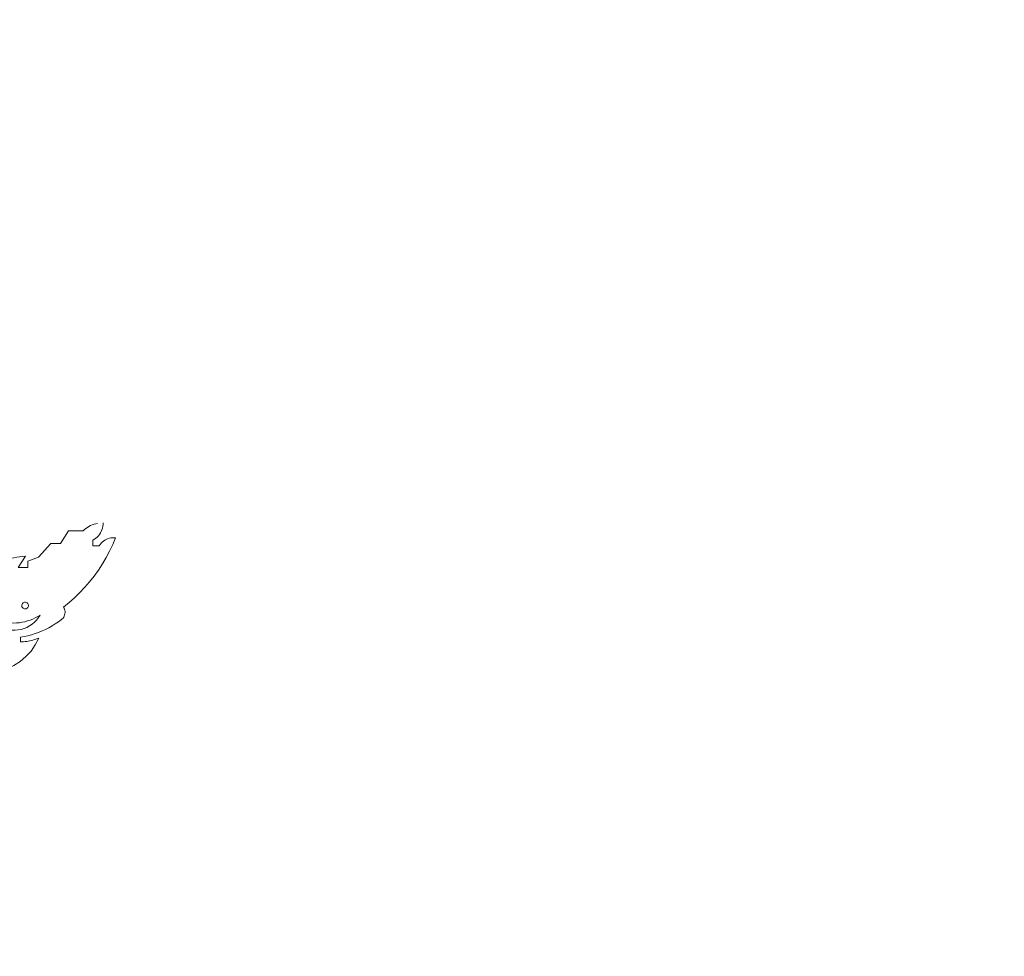
# Model space of a CAD drawing. Units: millimetres. Extents: x 7894 to 8038, y 6851 to 6951.
# Tile 26 of 49: x 7958.696 to 7966.961, y 6908.569 to 6916.434. Entities that reach past the tile are written whole.
import ezdxf

# ---------------------------------------------------------------- set-up
doc = ezdxf.new("R2010")
doc.units = ezdxf.units.MM
doc.layers.add('A-ANNO-DIMS', color=2, linetype='Continuous', lineweight=18)
doc.layers.add('A-FURN-ACCS', color=8, linetype='Continuous', lineweight=13)
doc.styles.get("Standard").update_dxf_attribs({"font": 'arial.ttf'})
doc.dimstyles.new('ISO-25', dxfattribs={"dimtxt": 1, "dimasz": 1, "dimexe": 1.25, "dimexo": 0.625, "dimtad": 1, "dimdec": 0, "dimlunit": 4, "dimtxsty": 'Standard', "dimcen": 2.5, "dimclrt": 1, "dimadec": 0, "dimazin": 0, "dimtfac": 1, "dimtdec": 0, "dimtmove": 0, "dimatfit": 3, "dimfxl": 1, "dimarcsym": 0})

# ---------------------------------------------------------------- blocks, each defined once
blk = doc.blocks.new('DISPLAY-LEAF-FINIAL')
for p, q in [((2.4341, 3.4699), (2.4472, 3.4778)), ((2.4472, 3.4778), (2.4609, 3.4849)), ((2.4609, 3.4849), (2.475, 3.4911)), ((2.475, 3.4911), (2.4894, 3.4964)), ((2.4894, 3.4964), (2.5041, 3.5007)), ((2.5041, 3.5007), (2.5191, 3.5041)), ((2.5634, 3.479), (2.5605, 3.4646)), ((2.5649, 3.4937), (2.5634, 3.479)), ((2.565, 3.5085), (2.5649, 3.4937)), ((2.2094, 3.3343), (2.2756, 3.4413)), ((2.2756, 3.4413), (2.398, 3.4413)), ((2.398, 3.4413), (2.4094, 3.4516)), ((2.4094, 3.4516), (2.4214, 3.4612)), ((2.4214, 3.4612), (2.4341, 3.4699)), ((2.5164, 3.3891), (2.5053, 3.3794)), ((2.5266, 3.3997), (2.5164, 3.3891)), ((2.5358, 3.4113), (2.5266, 3.3997)), ((2.5438, 3.4237), (2.5358, 3.4113)), ((2.5507, 3.4368), (2.5438, 3.4237)), ((2.5562, 3.4504), (2.5507, 3.4368)), ((2.5605, 3.4646), (2.5562, 3.4504)), ((2.0233, 3.2209), (2.1272, 3.3343)), ((2.1272, 3.3343), (2.2094, 3.3343)), ((2.4932, 3.3709), (2.4804, 3.3635)), ((2.4804, 3.3635), (2.4804, 3.3164)), ((2.4804, 3.3164), (2.5329, 3.3164)), ((2.5053, 3.3794), (2.4932, 3.3709)), ((2.5329, 3.3164), (2.5404, 3.3275)), ((2.5404, 3.3275), (2.5489, 3.3378)), ((2.5489, 3.3378), (2.5584, 3.3473)), ((2.5584, 3.3473), (2.5687, 3.3558)), ((2.5687, 3.3558), (2.5799, 3.3633)), ((2.5799, 3.3633), (2.5917, 3.3696)), ((2.5917, 3.3696), (2.604, 3.3748)), ((2.604, 3.3748), (2.6168, 3.3788)), ((2.6168, 3.3788), (2.63, 3.3815)), ((2.6462, 3.3254), (2.6199, 3.27)), ((2.63, 3.3815), (2.6433, 3.3829)), ((2.6433, 3.3829), (2.6567, 3.3831)), ((2.6701, 3.3819), (2.6462, 3.3254)), ((2.6567, 3.3831), (2.6701, 3.3819)), ((1.9139, 3.2271), (1.8536, 3.1329)), ((1.8651, 3.2232), (1.8895, 3.2256)), ((1.8895, 3.2256), (1.9139, 3.2271)), ((2.6199, 3.27), (2.5912, 3.2159)), ((1.3282, 3.1326), (1.3879, 3.1503)), ((1.3879, 3.1503), (1.4487, 3.1639)), ((1.4487, 3.1639), (1.5102, 3.1734)), ((1.5102, 3.1734), (1.5723, 3.1786)), ((1.5723, 3.1786), (1.5113, 3.0242)), ((1.5498, 3.0242), (1.6318, 3.1522)), ((1.6318, 3.1522), (1.6538, 3.163)), ((1.6538, 3.163), (1.6762, 3.173)), ((1.6762, 3.173), (1.6989, 3.1822)), ((1.6989, 3.1822), (1.7219, 3.1906)), ((1.7219, 3.1906), (1.7453, 3.1982)), ((1.7453, 3.1982), (1.7688, 3.2049)), ((1.7688, 3.2049), (1.7926, 3.2108)), ((1.7926, 3.2108), (1.8166, 3.2158)), ((1.8166, 3.2158), (1.8408, 3.2199)), ((1.8408, 3.2199), (1.8651, 3.2232)), ((1.934, 3.1854), (2.0233, 3.2209)), ((1.934, 3.1329), (1.934, 3.1854)), ((2.56, 3.1631), (2.5265, 3.1117)), ((2.5912, 3.2159), (2.56, 3.1631)), ((1.1581, 3.0558), (1.213, 3.0852)), ((1.213, 3.0852), (1.2698, 3.1109)), ((1.2698, 3.1109), (1.3282, 3.1326)), ((1.8536, 3.1329), (1.934, 3.1329)), ((2.4908, 3.0619), (2.4529, 3.0137)), ((2.5265, 3.1117), (2.4908, 3.0619)), ((1.0071, 2.9462), (1.0549, 2.9861)), ((1.0549, 2.9861), (1.1053, 3.0227)), ((1.1053, 3.0227), (1.1581, 3.0558)), ((1.5113, 3.0242), (1.5498, 3.0242)), ((2.4529, 3.0137), (2.4129, 2.9672)), ((0.634, 2.9001), (0.4633, 2.6089)), ((0.6052, 2.9243), (0.5471, 2.8395)), ((0.634, 2.9046), (0.5471, 2.8395)), ((0.634, 2.9046), (0.6052, 2.9243)), ((0.634, 2.9001), (0.634, 2.9046)), ((0.6629, 2.8848), (0.634, 2.9046)), ((0.9202, 2.857), (0.9622, 2.9031)), ((0.9622, 2.9031), (1.0071, 2.9462)), ((2.3708, 2.9226), (2.3268, 2.8799)), ((2.4129, 2.9672), (2.3708, 2.9226)), ((0.5471, 2.8395), (0.379, 2.7129)), ((0.5989, 2.7915), (0.6629, 2.8848)), ((0.9202, 2.857), (0.8844, 2.7861)), ((1.8829, 2.8172), (1.8849, 2.8243)), ((1.8829, 2.8099), (1.8829, 2.8172)), ((1.8849, 2.8243), (1.8885, 2.8306)), ((1.8885, 2.8306), (1.8937, 2.8357)), ((1.8937, 2.8357), (1.9001, 2.8393)), ((1.9001, 2.8393), (1.9071, 2.8412)), ((1.9071, 2.8412), (1.9144, 2.8411)), ((1.9144, 2.8411), (1.9215, 2.8392)), ((1.9215, 2.8392), (1.9278, 2.8355)), ((1.9278, 2.8355), (1.9329, 2.8303)), ((1.9329, 2.8303), (1.9365, 2.824)), ((1.9365, 2.824), (1.9384, 2.8169)), ((1.9384, 2.8169), (1.9383, 2.8096)), ((2.281, 2.8392), (2.2333, 2.8006)), ((2.3268, 2.8799), (2.281, 2.8392)), ((0.5406, 2.6956), (0.5989, 2.7915)), ((0.8844, 2.7861), (0.853, 2.7132)), ((1.8847, 2.8029), (1.8829, 2.8099)), ((1.8884, 2.7965), (1.8847, 2.8029)), ((1.8935, 2.7913), (1.8884, 2.7965)), ((1.8998, 2.7877), (1.8935, 2.7913)), ((1.9068, 2.7857), (1.8998, 2.7877)), ((1.9141, 2.7857), (1.9068, 2.7857)), ((1.9212, 2.7875), (1.9141, 2.7857)), ((1.9275, 2.7912), (1.9212, 2.7875)), ((1.9327, 2.7963), (1.9275, 2.7912)), ((1.9364, 2.8026), (1.9327, 2.7963)), ((1.9383, 2.8096), (1.9364, 2.8026)), ((2.0364, 2.7343), (2.0167, 2.7218)), ((2.0364, 2.7343), (2.023, 2.7124)), ((2.2333, 2.8006), (2.2382, 2.7921)), ((2.2382, 2.7921), (2.242, 2.7831)), ((2.243, 2.7351), (2.2397, 2.7259)), ((2.242, 2.7831), (2.2446, 2.7737)), ((2.2452, 2.7446), (2.243, 2.7351)), ((2.2446, 2.7737), (2.246, 2.764)), ((2.2462, 2.7543), (2.2452, 2.7446)), ((2.246, 2.764), (2.2462, 2.7543)), ((0.379, 2.7129), (0.2638, 2.6275)), ((0.3526, 2.6596), (0.3535, 2.675)), ((0.3527, 2.6591), (0.3526, 2.6596)), ((0.3526, 2.6569), (0.3527, 2.6591)), ((0.3535, 2.675), (0.3584, 2.6897)), ((0.3584, 2.6897), (0.3671, 2.7026)), ((0.3671, 2.7026), (0.379, 2.7129)), ((0.379, 2.7129), (0.3932, 2.7199)), ((0.3932, 2.7199), (0.4088, 2.7231)), ((0.4088, 2.7231), (0.4248, 2.7223)), ((0.4248, 2.7223), (0.44, 2.7176)), ((0.44, 2.7176), (0.4533, 2.7092)), ((0.4533, 2.7092), (0.464, 2.6977)), ((0.464, 2.6977), (0.4713, 2.6839)), ((0.4713, 2.6839), (0.4746, 2.6689)), ((0.4745, 2.6667), (0.4746, 2.6689)), ((0.4745, 2.6667), (0.4746, 2.6661)), ((0.5406, 2.6956), (0.4875, 2.5967)), ((0.853, 2.7132), (0.8261, 2.6384)), ((1.793, 2.6675), (1.7698, 2.6695)), ((1.7698, 2.6695), (1.7755, 2.6114)), ((1.8164, 2.6669), (1.793, 2.6675)), ((1.8397, 2.6677), (1.8164, 2.6669)), ((1.863, 2.6698), (1.8397, 2.6677)), ((1.886, 2.6733), (1.863, 2.6698)), ((1.9089, 2.6781), (1.886, 2.6733)), ((1.9314, 2.6843), (1.9089, 2.6781)), ((1.9535, 2.6918), (1.9314, 2.6843)), ((1.97, 2.6568), (1.9487, 2.6423)), ((1.9751, 2.7005), (1.9535, 2.6918)), ((1.9896, 2.6734), (1.97, 2.6568)), ((1.9962, 2.7106), (1.9751, 2.7005)), ((2.0073, 2.692), (1.9896, 2.6734)), ((2.0167, 2.7218), (1.9962, 2.7106)), ((2.023, 2.7124), (2.0073, 2.692)), ((2.1643, 2.6592), (2.1374, 2.6427)), ((2.1904, 2.6768), (2.1643, 2.6592)), ((2.2158, 2.6954), (2.1904, 2.6768)), ((2.2231, 2.7019), (2.2158, 2.6954)), ((2.2296, 2.7092), (2.2231, 2.7019)), ((2.2352, 2.7172), (2.2296, 2.7092)), ((2.2397, 2.7259), (2.2352, 2.7172)), ((0.2535, 2.6069), (0.2491, 2.5845)), ((0.2491, 2.58), (0.2491, 2.5845)), ((0.2491, 2.58), (0.2508, 2.5572)), ((0.2638, 2.6275), (0.2535, 2.6069)), ((0.4145, 2.6055), (0.4132, 2.6029)), ((0.4608, 2.6047), (0.4152, 2.527)), ((0.4402, 2.4957), (0.4858, 2.593)), ((0.4431, 2.613), (0.4459, 2.6117)), ((0.4509, 2.6151), (0.4489, 2.6161)), ((0.4633, 2.6089), (0.4608, 2.6047)), ((0.4858, 2.593), (0.4608, 2.6047)), ((0.4633, 2.6089), (0.4875, 2.5967)), ((0.8261, 2.6384), (0.804, 2.5621)), ((1.801, 2.6079), (1.7755, 2.6114)), ((1.8266, 2.607), (1.801, 2.6079)), ((1.8523, 2.6088), (1.8266, 2.607)), ((1.8776, 2.6133), (1.8523, 2.6088)), ((1.9023, 2.6204), (1.8776, 2.6133)), ((1.9261, 2.6301), (1.9023, 2.6204)), ((1.9487, 2.6423), (1.9261, 2.6301)), ((1.9641, 2.5686), (1.9336, 2.5606)), ((1.9942, 2.5779), (1.9641, 2.5686)), ((2.0239, 2.5884), (1.9942, 2.5779)), ((2.0531, 2.6002), (2.0239, 2.5884)), ((2.0818, 2.6131), (2.0531, 2.6002)), ((2.1099, 2.6273), (2.0818, 2.6131)), ((2.1374, 2.6427), (2.1099, 2.6273)), ((0.2508, 2.5572), (0.2586, 2.5356)), ((0.2586, 2.5356), (0.2719, 2.5167)), ((0.2719, 2.5167), (0.2898, 2.5018)), ((0.2898, 2.5018), (0.3111, 2.4919)), ((0.3111, 2.4919), (0.3343, 2.4876)), ((0.3628, 2.4909), (0.3323, 2.4155)), ((0.3343, 2.4876), (0.3579, 2.4893)), ((0.3579, 2.4893), (0.3628, 2.4909)), ((0.3628, 2.4909), (0.3802, 2.4968)), ((0.3649, 2.4962), (0.3628, 2.4909)), ((0.3802, 2.4968), (0.3998, 2.5097)), ((0.3978, 2.391), (0.4399, 2.495)), ((0.3983, 2.5132), (0.4016, 2.5117)), ((0.3998, 2.5097), (0.4016, 2.5117)), ((0.4029, 2.5132), (0.4004, 2.5144)), ((0.4016, 2.5117), (0.4029, 2.5132)), ((0.4016, 2.5117), (0.4399, 2.495)), ((0.4029, 2.5132), (0.4152, 2.527)), ((0.4029, 2.5132), (0.4402, 2.4957)), ((0.4085, 2.5106), (0.4078, 2.509)), ((0.4202, 2.5355), (0.4085, 2.5106)), ((0.7866, 2.4847), (0.774, 2.4062)), ((0.804, 2.5621), (0.7866, 2.4847)), ((1.9029, 2.5538), (1.8718, 2.5484)), ((1.8718, 2.5484), (1.8718, 2.5082)), ((1.8718, 2.5082), (1.885, 2.5088)), ((1.885, 2.5088), (1.8981, 2.5098)), ((1.8981, 2.5098), (1.9112, 2.5112)), ((1.9336, 2.5606), (1.9029, 2.5538)), ((1.9112, 2.5112), (1.9243, 2.513)), ((1.9243, 2.513), (1.9373, 2.5152)), ((1.9373, 2.5152), (1.9502, 2.5177)), ((1.9502, 2.5177), (1.9631, 2.5206)), ((1.9968, 2.4843), (1.9607, 2.4321)), ((1.9631, 2.5206), (1.9758, 2.5239)), ((1.9758, 2.5239), (1.9885, 2.5276)), ((1.9885, 2.5276), (2.001, 2.5317)), ((2.0257, 2.5409), (1.9968, 2.4843)), ((2.001, 2.5317), (2.0134, 2.5361)), ((2.0134, 2.5361), (2.0257, 2.5409)), ((0.3323, 2.4155), (0.2946, 2.3057)), ((0.774, 2.4062), (0.7662, 2.3272)), ((1.1631, 2.4165), (1.1364, 2.3787)), ((1.1928, 2.4521), (1.1631, 2.4165)), ((1.1981, 2.4572), (1.1928, 2.4521)), ((1.2041, 2.4615), (1.1981, 2.4572)), ((1.2106, 2.465), (1.2041, 2.4615)), ((1.2175, 2.4675), (1.2106, 2.465)), ((1.2247, 2.469), (1.2175, 2.4675)), ((1.2321, 2.4695), (1.2247, 2.469)), ((1.2395, 2.469), (1.2321, 2.4695)), ((1.2467, 2.4675), (1.2395, 2.469)), ((1.2536, 2.465), (1.2467, 2.4675)), ((1.2601, 2.4615), (1.2536, 2.465)), ((1.2661, 2.4572), (1.2601, 2.4615)), ((1.2714, 2.4521), (1.2661, 2.4572)), ((1.274, 2.435), (1.2714, 2.4521)), ((1.278, 2.4183), (1.274, 2.435)), ((1.2834, 2.4019), (1.278, 2.4183)), ((1.2903, 2.3861), (1.2834, 2.4019)), ((1.9607, 2.4321), (1.918, 2.3851)), ((0.3614, 2.2848), (0.3978, 2.391)), ((0.7662, 2.3272), (0.7634, 2.2478)), ((1.1127, 2.339), (1.0923, 2.2975)), ((1.1364, 2.3787), (1.1127, 2.339)), ((1.2985, 2.371), (1.2903, 2.3861)), ((1.308, 2.3566), (1.2985, 2.371)), ((1.3187, 2.3431), (1.308, 2.3566)), ((1.3305, 2.3306), (1.3187, 2.3431)), ((1.3434, 2.3192), (1.3305, 2.3306)), ((1.3572, 2.3089), (1.3434, 2.3192)), ((1.8695, 2.3441), (1.8161, 2.3099)), ((1.918, 2.3851), (1.8695, 2.3441)), ((0.2147, 2.201), (0.2202, 2.2445)), ((0.223, 2.2445), (0.2147, 2.201)), ((0.223, 2.2445), (0.2202, 2.2445)), ((0.223, 2.2445), (0.2299, 2.2445)), ((0.2325, 2.2195), (0.2299, 2.2445)), ((0.2946, 2.3057), (0.263, 2.1941)), ((0.3171, 2.2068), (0.3302, 2.2445)), ((0.3385, 2.2445), (0.3171, 2.2068)), ((0.3318, 2.2445), (0.3302, 2.2445)), ((0.3441, 2.2445), (0.3385, 2.2445)), ((0.3472, 2.2349), (0.3441, 2.2445)), ((0.3472, 2.2349), (0.3614, 2.2848)), ((0.3543, 2.2133), (0.3472, 2.2349)), ((0.5072, 2.2093), (0.5246, 2.2445)), ((0.5322, 2.2392), (0.5072, 2.2093)), ((0.5277, 2.2445), (0.5246, 2.2445)), ((0.5277, 2.2445), (0.5322, 2.2392)), ((0.5366, 2.2445), (0.5322, 2.2392)), ((0.5399, 2.2445), (0.5366, 2.2445)), ((0.5559, 2.2114), (0.5399, 2.2445)), ((0.7634, 2.2478), (0.7651, 2.1857)), ((0.8207, 2.2445), (0.7651, 2.1857)), ((0.93, 2.0453), (0.8207, 2.2445)), ((1.0703, 2.2388), (0.9394, 2.0859)), ((1.0703, 2.2388), (1.069, 2.2345)), ((1.0707, 2.2401), (1.0703, 2.2388)), ((1.0703, 2.2388), (1.0715, 2.2374)), ((1.0752, 2.2545), (1.0707, 2.2401)), ((1.0745, 2.2445), (1.0707, 2.2401)), ((1.0745, 2.2445), (1.0775, 2.2445)), ((1.0923, 2.2975), (1.0752, 2.2545)), ((1.0949, 2.2093), (1.0775, 2.2445)), ((1.2478, 2.2133), (1.2581, 2.2445)), ((1.2651, 2.2421), (1.2478, 2.2133)), ((1.2581, 2.2445), (1.2637, 2.2445)), ((1.2637, 2.2445), (1.2651, 2.2421)), ((1.2666, 2.2445), (1.2651, 2.2421)), ((1.2666, 2.2445), (1.272, 2.2445)), ((1.2851, 2.2068), (1.272, 2.2445)), ((1.3719, 2.2999), (1.3572, 2.3089)), ((1.3697, 2.2195), (1.3722, 2.2445)), ((1.3751, 2.2445), (1.3697, 2.2195)), ((1.3873, 2.2921), (1.3719, 2.2999)), ((1.3722, 2.2445), (1.3751, 2.2445)), ((1.3751, 2.2445), (1.3819, 2.2445)), ((1.3819, 2.2445), (1.3889, 2.1901)), ((1.4469, 2.2701), (1.3873, 2.2921)), ((1.5088, 2.256), (1.4469, 2.2701)), ((1.572, 2.2503), (1.5088, 2.256)), ((1.6355, 2.2529), (1.572, 2.2503)), ((1.698, 2.2639), (1.6355, 2.2529)), ((1.7585, 2.283), (1.698, 2.2639)), ((1.8161, 2.3099), (1.7585, 2.283)), ((0.2133, 2.1901), (0.1946, 2.0859)), ((0.2133, 2.1901), (0.2147, 2.201)), ((0.2325, 2.2195), (0.2504, 2.1381)), ((0.2439, 2.1095), (0.2325, 2.2195)), ((0.3171, 2.2068), (0.2485, 2.0859)), ((0.263, 2.1941), (0.2504, 2.1381)), ((0.2969, 2.1855), (0.2916, 2.1618)), ((0.3543, 2.2133), (0.4197, 2.1042)), ((0.4044, 2.0607), (0.3543, 2.2133)), ((0.5072, 2.2093), (0.4197, 2.1042)), ((0.5482, 2.2204), (0.5559, 2.2114)), ((0.5559, 2.2114), (0.6628, 2.0859)), ((0.636, 2.0453), (0.5559, 2.2114)), ((0.7651, 2.1857), (0.6705, 2.0859)), ((1.0949, 2.2093), (1.1824, 2.1042)), ((1.0949, 2.2093), (1.1714, 2.0542)), ((1.2478, 2.2133), (1.1824, 2.1042)), ((1.2851, 2.2068), (1.3441, 2.1028)), ((1.2851, 2.2068), (1.3403, 2.0478)), ((1.3697, 2.2195), (1.3441, 2.1028)), ((1.3889, 2.1901), (1.4075, 2.0859)), ((1.4073, 2.0453), (1.3889, 2.1901)), ((0.1946, 2.0859), (0.1952, 2.0478)), ((0.2439, 2.1095), (0.2392, 2.0887)), ((0.2504, 2.1381), (0.2439, 2.1095)), ((0.2485, 2.0654), (0.2439, 2.1095)), ((0.2485, 2.0859), (0.2485, 2.0654)), ((0.2504, 2.1381), (0.2555, 2.1145)), ((0.4197, 2.1042), (0.4044, 2.0859)), ((0.4044, 2.0859), (0.4044, 2.0607)), ((0.6628, 2.0859), (0.6628, 1.9035)), ((0.6705, 2.0859), (0.6705, 1.9035)), ((0.9394, 2.0859), (0.9394, 1.9343)), ((1.1824, 2.1042), (1.1714, 2.0859)), ((1.1714, 2.0859), (1.1714, 2.0542)), ((1.3441, 2.1028), (1.3403, 2.0859)), ((1.3403, 2.0859), (1.3403, 2.0478)), ((1.4075, 2.0859), (1.4073, 2.0453)), ((0.1949, 2.0453), (0.1946, 1.903)), ((0.1949, 2.0453), (0.1952, 2.0478)), ((0.211, 1.9837), (0.2126, 1.986)), ((0.2161, 1.986), (0.2126, 1.986)), ((0.2144, 1.9837), (0.2161, 1.986)), ((0.2485, 2.0654), (0.2485, 1.9035)), ((0.3083, 1.9837), (0.3136, 1.986)), ((0.3164, 1.986), (0.3136, 1.986)), ((0.4044, 2.0607), (0.4044, 1.9015)), ((0.4947, 1.9837), (0.5025, 1.986)), ((0.5041, 1.986), (0.5025, 1.986)), ((0.636, 2.0453), (0.6371, 1.9035)), ((0.775, 1.9837), (0.7838, 1.986)), ((0.7838, 1.986), (0.793, 1.986)), ((0.793, 1.986), (0.8018, 1.9836)), ((0.93, 2.0453), (0.9309, 1.9342)), ((1.0443, 1.986), (1.0459, 1.986)), ((1.0459, 1.986), (1.0541, 1.986)), ((1.0541, 1.986), (1.062, 1.9836)), ((1.1758, 2.0453), (1.1714, 2.0542)), ((1.1758, 2.0453), (1.1768, 1.9142)), ((1.2486, 1.986), (1.2513, 1.986)), ((1.2513, 1.986), (1.2571, 1.986)), ((1.2571, 1.986), (1.2627, 1.9836)), ((1.3412, 2.0453), (1.3403, 2.0478)), ((1.3412, 2.0453), (1.342, 1.9035)), ((1.3734, 1.986), (1.3755, 1.986)), ((1.3755, 1.986), (1.3775, 1.9836)), ((1.3755, 1.986), (1.3768, 1.986)), ((1.3768, 1.986), (1.3789, 1.986)), ((1.3789, 1.986), (1.3809, 1.9836)), ((1.4073, 2.0453), (1.4075, 1.903)), ((0.1817, 1.8976), (0.1887, 1.9015)), ((0.1887, 1.9015), (0.1946, 1.903)), ((0.1946, 1.903), (0.1964, 1.9035)), ((0.1946, 1.903), (0.1946, 1.9015)), ((0.1964, 1.9035), (0.1977, 1.9034)), ((0.1964, 1.9035), (0.1969, 1.9035)), ((0.2373, 1.9035), (0.1977, 1.9034)), ((0.2069, 1.956), (0.2074, 1.9648)), ((0.2069, 1.9469), (0.2069, 1.956)), ((0.2074, 1.938), (0.2069, 1.9469)), ((0.2074, 1.9648), (0.2082, 1.9727)), ((0.2082, 1.9301), (0.2074, 1.938)), ((0.2082, 1.9727), (0.2095, 1.9791)), ((0.2094, 1.9236), (0.2082, 1.9301)), ((0.2109, 1.9191), (0.2094, 1.9236)), ((0.2095, 1.9791), (0.211, 1.9837)), ((0.2103, 1.9469), (0.2104, 1.956)), ((0.2108, 1.938), (0.2103, 1.9469)), ((0.2104, 1.956), (0.2108, 1.9648)), ((0.2108, 1.9648), (0.2117, 1.9727)), ((0.2116, 1.9301), (0.2108, 1.938)), ((0.2126, 1.9167), (0.2109, 1.9191)), ((0.2129, 1.9236), (0.2116, 1.9301)), ((0.2117, 1.9727), (0.2129, 1.9791)), ((0.2143, 1.9167), (0.2126, 1.9167)), ((0.2129, 1.9791), (0.2144, 1.9837)), ((0.2163, 1.9467), (0.2129, 1.9236)), ((0.2144, 1.9191), (0.2129, 1.9236)), ((0.216, 1.9167), (0.2143, 1.9167)), ((0.216, 1.9167), (0.2144, 1.9191)), ((0.2177, 1.9167), (0.216, 1.9167)), ((0.2168, 1.9646), (0.2163, 1.9558)), ((0.2163, 1.9558), (0.2163, 1.9467)), ((0.2163, 1.9467), (0.2168, 1.9379)), ((0.2179, 1.9725), (0.2168, 1.9646)), ((0.218, 1.9665), (0.2168, 1.9646)), ((0.2168, 1.9379), (0.2179, 1.93)), ((0.2194, 1.979), (0.2179, 1.9725)), ((0.2179, 1.9725), (0.218, 1.9665)), ((0.2179, 1.93), (0.2194, 1.9235)), ((0.2202, 1.9812), (0.2194, 1.979)), ((0.2204, 1.9806), (0.2194, 1.979)), ((0.2194, 1.9235), (0.2202, 1.9215)), ((0.2202, 1.9646), (0.2197, 1.9558)), ((0.2197, 1.9558), (0.2197, 1.9467)), ((0.2197, 1.9467), (0.2202, 1.9379)), ((0.2213, 1.9725), (0.2202, 1.9646)), ((0.2202, 1.9379), (0.2213, 1.93)), ((0.2218, 1.9746), (0.2213, 1.9725)), ((0.2213, 1.93), (0.2218, 1.928)), ((0.2485, 1.9035), (0.2439, 1.9035)), ((0.2485, 1.9251), (0.2458, 1.9015)), ((0.2485, 1.9035), (0.2485, 1.9015)), ((0.3913, 1.9035), (0.265, 1.9035)), ((0.2955, 1.956), (0.2969, 1.9648)), ((0.2955, 1.9469), (0.2955, 1.956)), ((0.2969, 1.938), (0.2955, 1.9469)), ((0.2969, 1.9648), (0.2997, 1.9727)), ((0.2996, 1.9301), (0.2969, 1.938)), ((0.3034, 1.9236), (0.2996, 1.9301)), ((0.2997, 1.9727), (0.3035, 1.9791)), ((0.3082, 1.9191), (0.3034, 1.9236)), ((0.3035, 1.9791), (0.3083, 1.9837)), ((0.3134, 1.9167), (0.3082, 1.9191)), ((0.3189, 1.9167), (0.3134, 1.9167)), ((0.3217, 1.9167), (0.3189, 1.9167)), ((0.4385, 1.9035), (0.6066, 1.9035)), ((0.4759, 1.956), (0.478, 1.9648)), ((0.4759, 1.9469), (0.4759, 1.956)), ((0.478, 1.938), (0.4759, 1.9469)), ((0.478, 1.9648), (0.482, 1.9727)), ((0.4819, 1.9301), (0.478, 1.938)), ((0.4876, 1.9236), (0.4819, 1.9301)), ((0.482, 1.9727), (0.4877, 1.9791)), ((0.4945, 1.9191), (0.4876, 1.9236)), ((0.4877, 1.9791), (0.4947, 1.9837)), ((0.5023, 1.9167), (0.4945, 1.9191)), ((0.5103, 1.9167), (0.5023, 1.9167)), ((0.512, 1.9167), (0.5103, 1.9167)), ((0.6371, 1.9035), (0.6338, 1.9035)), ((0.6371, 1.9035), (0.6371, 1.9015)), ((0.6628, 1.9035), (0.6371, 1.9035)), ((0.6628, 1.9035), (0.6705, 1.9035)), ((0.6628, 1.9035), (0.6628, 1.9015)), ((0.6705, 1.9035), (0.6705, 1.9015)), ((0.7081, 1.9035), (0.894, 1.9035)), ((0.7536, 1.9469), (0.7537, 1.956)), ((0.756, 1.938), (0.7536, 1.9469)), ((0.7537, 1.956), (0.756, 1.9648)), ((0.756, 1.9648), (0.7606, 1.9727)), ((0.7605, 1.9301), (0.756, 1.938)), ((0.7669, 1.9236), (0.7605, 1.9301)), ((0.7606, 1.9727), (0.7671, 1.9791)), ((0.7748, 1.9191), (0.7669, 1.9236)), ((0.7671, 1.9791), (0.775, 1.9837)), ((0.7836, 1.9167), (0.7748, 1.9191)), ((0.7928, 1.9167), (0.7836, 1.9167)), ((0.8016, 1.919), (0.7928, 1.9167)), ((0.8095, 1.9235), (0.8016, 1.919)), ((0.8018, 1.9836), (0.8096, 1.979)), ((0.816, 1.93), (0.8095, 1.9235)), ((0.8096, 1.979), (0.8161, 1.9725)), ((0.8206, 1.9379), (0.816, 1.93)), ((0.8161, 1.9725), (0.8206, 1.9646)), ((0.8206, 1.9646), (0.823, 1.9558)), ((0.8229, 1.9467), (0.8206, 1.9379)), ((0.823, 1.9558), (0.8229, 1.9467)), ((0.9394, 1.9343), (0.9309, 1.9342)), ((0.9309, 1.9342), (0.9312, 1.9035)), ((0.9312, 1.9035), (0.9312, 1.9015)), ((0.9394, 1.9035), (0.9312, 1.9035)), ((0.9424, 1.9343), (0.9394, 1.9343)), ((0.9394, 1.9343), (0.9394, 1.9035)), ((0.9424, 1.9035), (0.9394, 1.9035)), ((0.9394, 1.9035), (0.9394, 1.9015)), ((0.9534, 1.9035), (1.1456, 1.9035)), ((1.0224, 1.935), (1.0209, 1.935)), ((1.0524, 1.9167), (1.0539, 1.9167)), ((1.0618, 1.919), (1.0539, 1.9167)), ((1.069, 1.9235), (1.0618, 1.919)), ((1.062, 1.9836), (1.0691, 1.979)), ((1.0748, 1.93), (1.069, 1.9235)), ((1.0691, 1.979), (1.0749, 1.9725)), ((1.0789, 1.9379), (1.0748, 1.93)), ((1.0749, 1.9725), (1.079, 1.9646)), ((1.0811, 1.9467), (1.0789, 1.9379)), ((1.079, 1.9646), (1.0811, 1.9558)), ((1.0811, 1.9558), (1.0811, 1.9467)), ((1.3304, 1.9035), (1.1965, 1.9035)), ((1.2543, 1.9167), (1.257, 1.9167)), ((1.2626, 1.919), (1.257, 1.9167)), ((1.2676, 1.9235), (1.2626, 1.919)), ((1.2627, 1.9836), (1.2677, 1.979)), ((1.2717, 1.93), (1.2676, 1.9235)), ((1.2677, 1.979), (1.2717, 1.9725)), ((1.2717, 1.9725), (1.2746, 1.9646)), ((1.2746, 1.9379), (1.2717, 1.93)), ((1.2746, 1.9646), (1.2761, 1.9558)), ((1.2761, 1.9467), (1.2746, 1.9379)), ((1.2761, 1.9558), (1.2761, 1.9467)), ((1.3471, 1.9035), (1.342, 1.9035)), ((1.342, 1.9035), (1.342, 1.9015)), ((1.3561, 1.9035), (1.4004, 1.9035)), ((1.3775, 1.919), (1.3755, 1.9167)), ((1.3755, 1.9167), (1.3789, 1.9167)), ((1.3775, 1.9836), (1.3794, 1.979)), ((1.3793, 1.9235), (1.3775, 1.919)), ((1.3809, 1.919), (1.3789, 1.9167)), ((1.3808, 1.93), (1.3793, 1.9235)), ((1.3794, 1.979), (1.3809, 1.9725)), ((1.3819, 1.9379), (1.3808, 1.93)), ((1.3809, 1.9836), (1.3828, 1.979)), ((1.3809, 1.9725), (1.3819, 1.9646)), ((1.3827, 1.9235), (1.3809, 1.919)), ((1.3819, 1.9646), (1.3825, 1.9558)), ((1.3825, 1.9467), (1.3819, 1.9379)), ((1.3825, 1.9558), (1.3825, 1.9467)), ((1.3842, 1.93), (1.3827, 1.9235)), ((1.3828, 1.979), (1.3843, 1.9725)), ((1.3853, 1.9379), (1.3842, 1.93)), ((1.3843, 1.9725), (1.3853, 1.9646)), ((1.3853, 1.9646), (1.3859, 1.9558)), ((1.3859, 1.9467), (1.3853, 1.9379)), ((1.3859, 1.9558), (1.3859, 1.9467)), ((1.4075, 1.903), (1.4135, 1.9015)), ((1.4075, 1.903), (1.4075, 1.9015)), ((1.4135, 1.9015), (1.4205, 1.8976)), ((0, 1.6201), (0.181, 1.8491)), ((0.1696, 1.8695), (0.1697, 1.8775)), ((0.1715, 1.8618), (0.1696, 1.8695)), ((0.1697, 1.8775), (0.1719, 1.8852)), ((0.1754, 1.8548), (0.1715, 1.8618)), ((0.1719, 1.8852), (0.176, 1.892)), ((0.181, 1.8491), (0.1754, 1.8548)), ((0.176, 1.892), (0.1817, 1.8976)), ((0.1946, 1.8976), (0.1945, 1.8695)), ((0.1945, 1.8618), (0.1945, 1.8548)), ((0.1952, 1.8548), (0.1945, 1.8548)), ((0.2052, 1.8548), (0.1945, 1.8548)), ((0.2048, 1.8513), (0.2047, 1.8491)), ((0.2052, 1.8548), (0.2048, 1.8513)), ((0.2485, 1.8548), (0.2052, 1.8548)), ((0.2404, 1.8548), (0.2398, 1.8491)), ((0.2485, 1.8971), (0.2439, 1.8971)), ((0.2453, 1.8976), (0.244, 1.8856)), ((0.2485, 1.8976), (0.2485, 1.8971)), ((0.2485, 1.8971), (0.2485, 1.8695)), ((0.2485, 1.8618), (0.2485, 1.8548)), ((0.2485, 1.8548), (0.2756, 1.8548)), ((0.275, 1.8491), (0.2756, 1.8548)), ((0.2756, 1.8548), (0.4049, 1.8548)), ((0.4044, 1.8976), (0.4044, 1.8695)), ((0.4044, 1.8618), (0.4049, 1.8548)), ((0.4049, 1.8548), (0.6375, 1.8548)), ((0.6371, 1.8971), (0.6338, 1.8971)), ((0.6371, 1.8976), (0.6371, 1.8971)), ((0.6371, 1.8971), (0.6374, 1.8695)), ((0.6628, 1.8971), (0.6371, 1.8971)), ((0.6374, 1.8618), (0.6375, 1.8548)), ((0.6628, 1.8548), (0.6375, 1.8548)), ((0.6628, 1.8976), (0.6628, 1.8971)), ((0.6628, 1.8971), (0.6628, 1.8695)), ((0.6705, 1.8971), (0.6628, 1.8971)), ((0.6628, 1.8618), (0.6628, 1.8548)), ((0.6705, 1.8976), (0.6705, 1.8971)), ((0.6705, 1.8971), (0.6705, 1.8695)), ((0.6705, 1.8618), (0.6705, 1.8548)), ((0.6705, 1.8548), (0.9316, 1.8548)), ((0.9313, 1.8976), (0.9313, 1.8971)), ((0.9313, 1.8971), (0.9315, 1.8695)), ((0.9394, 1.8971), (0.9313, 1.8971)), ((0.9316, 1.8618), (0.9316, 1.8548)), ((0.9394, 1.8548), (0.9316, 1.8548)), ((0.9394, 1.8976), (0.9394, 1.8971)), ((0.9424, 1.8971), (0.9394, 1.8971)), ((0.9394, 1.8971), (0.9394, 1.8695)), ((0.9394, 1.8618), (0.9394, 1.8548)), ((1.3422, 1.8548), (0.9394, 1.8548)), ((1.342, 1.8976), (1.342, 1.8971)), ((1.3471, 1.8971), (1.342, 1.8971)), ((1.342, 1.8971), (1.3421, 1.8695)), ((1.3422, 1.8618), (1.3422, 1.8548)), ((1.4075, 1.8548), (1.3422, 1.8548)), ((1.4075, 1.8976), (1.4075, 1.8695)), ((1.4075, 1.8618), (1.4075, 1.8548)), ((1.4205, 1.8976), (1.4262, 1.892)), ((1.4267, 1.8548), (1.4212, 1.8491)), ((1.4212, 1.8491), (1.6021, 1.6201)), ((1.4262, 1.892), (1.4303, 1.8852)), ((1.4306, 1.8618), (1.4267, 1.8548)), ((1.4303, 1.8852), (1.4325, 1.8775)), ((1.4326, 1.8695), (1.4306, 1.8618)), ((1.4325, 1.8775), (1.4326, 1.8695)), ((0.2072, 1.3429), (0, 1.6201)), ((1.6021, 1.6201), (0, 1.6201)), ((1.6021, 1.6201), (1.395, 1.3429)), ((0.1742, 1.3213), (0.1833, 1.3311)), ((0.1833, 1.3311), (0.1945, 1.3384)), ((0.1945, 1.3384), (0.2072, 1.3429)), ((1.395, 1.3429), (1.4076, 1.3384)), ((1.4076, 1.3384), (1.4188, 1.3311)), ((1.4188, 1.3311), (1.4279, 1.3213)), ((0.1641, 1.2831), (0.1643, 1.2966)), ((0.1672, 1.2701), (0.1641, 1.2831)), ((0.1643, 1.2966), (0.1678, 1.3095)), ((0.1733, 1.2582), (0.1672, 1.2701)), ((0.1678, 1.3095), (0.1742, 1.3213)), ((0.1821, 1.2481), (0.1733, 1.2582)), ((0.1931, 1.2404), (0.1821, 1.2481)), ((0.2056, 1.2356), (0.1931, 1.2404)), ((1.4091, 1.2404), (1.3965, 1.2356)), ((1.42, 1.2481), (1.4091, 1.2404)), ((1.4288, 1.2582), (1.42, 1.2481)), ((1.4279, 1.3213), (1.4344, 1.3095)), ((1.435, 1.2701), (1.4288, 1.2582)), ((1.4344, 1.3095), (1.4378, 1.2966)), ((1.438, 1.2831), (1.435, 1.2701)), ((1.4378, 1.2966), (1.438, 1.2831)), ((0.1714, 0.9553), (0.1907, 1.234)), ((0.2189, 1.234), (0.1907, 1.234)), ((0.1964, 0.9543), (0.3109, 1.2098)), ((0.2018, 1.1515), (0.2065, 1.165)), ((0.2189, 1.234), (0.2056, 1.2356)), ((0.2065, 1.165), (0.2118, 1.177)), ((0.2118, 1.177), (0.2173, 1.1867)), ((0.2147, 0.949), (0.3244, 1.1717)), ((0.2173, 1.1867), (0.2227, 1.1934)), ((0.2189, 1.234), (0.2969, 1.234)), ((0.2227, 1.1934), (0.2276, 1.1967)), ((0.2276, 1.1967), (0.2317, 1.1963)), ((0.2325, 1.1953), (0.2317, 1.1963)), ((0.2325, 1.1953), (0.2366, 1.1949)), ((0.2969, 1.234), (0.3023, 1.234)), ((0.3029, 1.2321), (0.2969, 1.234)), ((0.3029, 1.2321), (0.3023, 1.234)), ((0.3023, 1.234), (0.5943, 1.234)), ((0.3109, 1.2098), (0.3029, 1.2321)), ((0.3244, 1.1717), (0.3109, 1.2098)), ((0.4015, 0.9553), (0.3244, 1.1717)), ((0.3893, 1.1515), (0.3948, 1.165)), ((0.3948, 1.165), (0.4028, 1.177)), ((0.4028, 1.177), (0.4128, 1.1867)), ((0.4128, 1.1867), (0.4241, 1.1934)), ((0.4241, 1.1934), (0.436, 1.1967)), ((0.434, 0.9751), (0.6087, 1.2276)), ((0.436, 1.1967), (0.4475, 1.1963)), ((0.4475, 1.1963), (0.4584, 1.1919)), ((0.455, 0.949), (0.6322, 1.205)), ((0.4584, 1.1919), (0.4611, 1.1909)), ((0.5943, 1.234), (0.6175, 1.234)), ((0.6087, 1.2276), (0.5943, 1.234)), ((0.6175, 1.2276), (0.6175, 1.234)), ((0.9517, 1.234), (0.6175, 1.234)), ((0.6322, 1.205), (0.6175, 1.2276)), ((0.7416, 1.0372), (0.6322, 1.205)), ((0.7478, 1.1515), (0.752, 1.165)), ((0.752, 1.165), (0.7597, 1.177)), ((0.7597, 1.177), (0.7703, 1.1867)), ((0.7703, 1.1867), (0.7831, 1.1934)), ((0.7831, 1.1934), (0.7973, 1.1967)), ((0.7973, 1.1967), (0.8119, 1.1963)), ((0.8119, 1.1963), (0.8259, 1.1923)), ((0.8259, 1.1923), (0.8383, 1.1849)), ((0.8383, 1.1849), (0.8484, 1.1746)), ((0.8484, 1.1746), (0.8553, 1.1622)), ((0.8553, 1.1622), (0.8587, 1.1485)), ((0.8605, 1.0411), (0.9765, 1.2154)), ((0.8605, 0.9923), (0.9902, 1.1955)), ((0.9809, 1.2337), (0.9517, 1.234)), ((0.9765, 1.2154), (0.9744, 1.2185)), ((0.9902, 1.1955), (0.9765, 1.2154)), ((0.9809, 1.2337), (0.9815, 1.234)), ((0.9815, 1.234), (0.983, 1.234)), ((1.2836, 1.234), (0.983, 1.234)), ((1.16, 0.949), (0.9902, 1.1955)), ((1.1241, 1.1921), (1.1257, 1.1925)), ((1.1257, 1.1925), (1.127, 1.1934)), ((1.127, 1.1934), (1.1382, 1.1967)), ((1.1382, 1.1967), (1.1502, 1.1963)), ((1.1502, 1.1963), (1.1624, 1.1923)), ((1.1624, 1.1923), (1.1737, 1.1849)), ((1.1737, 1.1849), (1.1835, 1.1746)), ((1.1768, 0.964), (1.2748, 1.2121)), ((1.1835, 1.1746), (1.1911, 1.1622)), ((1.1911, 1.1622), (1.196, 1.1485)), ((1.2015, 0.9553), (1.285, 1.1903)), ((1.2748, 1.2121), (1.2826, 1.2319)), ((1.285, 1.1903), (1.2748, 1.2121)), ((1.2826, 1.2319), (1.2898, 1.234)), ((1.2826, 1.2319), (1.2836, 1.234)), ((1.2836, 1.234), (1.2898, 1.234)), ((1.398, 0.949), (1.285, 1.1903)), ((1.2898, 1.234), (1.3832, 1.234)), ((1.359, 1.1953), (1.3638, 1.1967)), ((1.359, 1.1953), (1.3619, 1.1951)), ((1.3638, 1.1967), (1.3687, 1.1963)), ((1.3687, 1.1963), (1.3744, 1.1923)), ((1.3744, 1.1923), (1.3804, 1.1849)), ((1.3804, 1.1849), (1.3863, 1.1746)), ((1.3965, 1.2356), (1.3832, 1.234)), ((1.41, 1.2337), (1.3832, 1.234)), ((1.3863, 1.1746), (1.3917, 1.1622)), ((1.3917, 1.1622), (1.3963, 1.1485)), ((1.4111, 1.234), (1.41, 1.2337)), ((1.4113, 1.2316), (1.4111, 1.234)), ((1.4348, 0.9553), (1.4113, 1.2316)), ((1.4203, 0.9553), (1.4113, 1.2316)), ((0.1943, 1.1113), (0.1955, 1.1237)), ((0.1946, 1.101), (0.1943, 1.1113)), ((0.1963, 1.0936), (0.1946, 1.101)), ((0.1955, 1.1237), (0.1981, 1.1374)), ((0.1993, 1.0896), (0.1963, 1.0936)), ((0.1981, 1.1374), (0.2018, 1.1515)), ((0.2034, 1.0892), (0.1993, 1.0896)), ((0.2041, 1.0883), (0.2034, 1.0892)), ((0.2112, 1.0961), (0.2129, 1.0925)), ((0.2129, 1.0925), (0.2137, 1.0919)), ((0.2141, 1.1), (0.2145, 1.0978)), ((0.3867, 1.1374), (0.3893, 1.1515)), ((0.3871, 1.1237), (0.3867, 1.1374)), ((0.3906, 1.1113), (0.3871, 1.1237)), ((0.3969, 1.101), (0.3906, 1.1113)), ((0.4056, 1.0936), (0.3969, 1.101)), ((0.4087, 1.0923), (0.4056, 1.0936)), ((0.7474, 1.1361), (0.7475, 1.1373)), ((0.7475, 1.1373), (0.7478, 1.1515)), ((0.8587, 1.1471), (0.8587, 1.1485)), ((1.1736, 1.092), (1.1723, 1.0911)), ((1.1736, 1.092), (1.1752, 1.0925)), ((1.1847, 1.0992), (1.1752, 1.0925)), ((1.192, 1.1089), (1.1847, 1.0992)), ((1.1964, 1.1209), (1.192, 1.1089)), ((1.196, 1.1485), (1.1978, 1.1344)), ((1.1978, 1.1344), (1.1964, 1.1209)), ((1.3919, 1.0894), (1.39, 1.0879)), ((1.39, 1.0879), (1.3948, 1.0892)), ((1.3987, 1.0925), (1.3948, 1.0892)), ((1.3963, 1.1485), (1.3997, 1.1344)), ((1.4012, 1.0992), (1.3987, 1.0925)), ((1.3997, 1.1344), (1.4018, 1.1209)), ((1.4023, 1.1089), (1.4012, 1.0992)), ((1.4018, 1.1209), (1.4023, 1.1089)), ((0.7416, 0), (0.7416, 1.0372)), ((0.7992, 0.949), (0.7416, 1.0372)), ((0.8158, 0.974), (0.8605, 1.0411)), ((0.8431, 0.9651), (0.8605, 0.9923)), ((0.8605, 1.0411), (0.8605, 1.0475)), ((0.8605, 0.9923), (0.8605, 1.0411)), ((0.8605, 0), (0.8605, 0.9923)), ((0.1941, 0.949), (0.1714, 0.9553)), ((0.1941, 0.949), (0.1964, 0.9543)), ((0.2147, 0.949), (0.1964, 0.9543)), ((0.4159, 0.949), (0.4015, 0.9553)), ((0.4159, 0.949), (0.434, 0.9751)), ((0.4421, 0.9553), (0.434, 0.9751)), ((0.455, 0.949), (0.4421, 0.9553)), ((0.7992, 0.949), (0.8158, 0.974)), ((0.8158, 0.974), (0.8137, 0.9772)), ((0.8165, 0.9731), (0.8158, 0.974)), ((1.16, 0.949), (1.1734, 0.9553)), ((1.1734, 0.9553), (1.1768, 0.964)), ((1.1872, 0.949), (1.1768, 0.964)), ((1.1872, 0.949), (1.2015, 0.9553)), ((1.398, 0.949), (1.4105, 0.9525)), ((1.4105, 0.9525), (1.4203, 0.9553)), ((1.412, 0.949), (1.4105, 0.9525)), ((1.412, 0.949), (1.4348, 0.9553))]:
    blk.add_line(p, q)
blk = doc.blocks.new('*D23')
at = {"layer": 'A-ANNO-DIMS', "color": 0, "lineweight": -2, "transparency": 16777216}
for p, q in [((7940.0888, 6907.098), (7940.0888, 6947.7928)), ((7971.9356, 6928.989), (7971.9356, 6947.7928)), ((7941.0888, 6946.5428), (7970.9356, 6946.5428))]:
    blk.add_line(p, q, dxfattribs=at)
at = {"layer": 'A-ANNO-DIMS', "color": 0, "transparency": 16777216}
for points in [[(7941.0888, 6946.7095), (7941.0888, 6946.3762), (7940.0888, 6946.5428)], [(7970.9356, 6946.7095), (7970.9356, 6946.3762), (7971.9356, 6946.5428)]]:
    blk.add_solid(points, dxfattribs=at)
at = {"layer": 'Defpoints', "color": 0, "transparency": 16777216}
for p in [(7971.9356, 6946.5428), (7971.9356, 6928.364), (7940.0888, 6906.473)]:
    blk.add_point(p, dxfattribs=at)
at = {"layer": 'A-ANNO-DIMS', "color": 1, "transparency": 16777216, "insert": (7956.0122, 6947.6784), "char_height": 1, "attachment_point": 5}
blk.add_mtext('2\'-8"', dxfattribs=at)
blk = doc.blocks.new('*D26')
at = {"layer": 'A-ANNO-DIMS', "color": 0, "lineweight": -2, "transparency": 16777216}
for p, q in [((7950.9654, 6918.7198), (7975.2272, 6918.7198)), ((7973.9772, 6917.7198), (7973.9772, 6907.4734)), ((7964.9658, 6906.4734), (7975.2272, 6906.4734))]:
    blk.add_line(p, q, dxfattribs=at)
at = {"layer": 'A-ANNO-DIMS', "color": 0, "transparency": 16777216}
for points in [[(7973.8105, 6917.7198), (7974.1439, 6917.7198), (7973.9772, 6918.7198)], [(7973.8105, 6907.4734), (7974.1439, 6907.4734), (7973.9772, 6906.4734)]]:
    blk.add_solid(points, dxfattribs=at)
at = {"layer": 'Defpoints', "color": 0, "transparency": 16777216}
for p in [(7950.3404, 6918.7198), (7964.3408, 6906.4734), (7973.9772, 6906.4734)]:
    blk.add_point(p, dxfattribs=at)
at = {"layer": 'A-ANNO-DIMS', "color": 1, "transparency": 16777216, "insert": (7972.8416, 6912.5966), "char_height": 1, "attachment_point": 5, "rotation": 90}
blk.add_mtext('1\'-0"', dxfattribs=at)
blk = doc.blocks.new('*D34')
at = {"layer": 'A-ANNO-DIMS', "color": 0, "lineweight": -2, "transparency": 16777216}
for p, q in [((7971.2171, 6922.0033), (7971.2171, 6903.2865)), ((7964.3408, 6905.8484), (7964.3408, 6903.2865)), ((7965.3408, 6904.5365), (7970.2171, 6904.5365))]:
    blk.add_line(p, q, dxfattribs=at)
at = {"layer": 'A-ANNO-DIMS', "color": 0, "transparency": 16777216}
for points in [[(7965.3408, 6904.7032), (7965.3408, 6904.3699), (7964.3408, 6904.5365)], [(7970.2171, 6904.7032), (7970.2171, 6904.3699), (7971.2171, 6904.5365)]]:
    blk.add_solid(points, dxfattribs=at)
at = {"layer": 'Defpoints', "color": 0, "transparency": 16777216}
for p in [(7971.2171, 6922.6283), (7964.3408, 6906.4734), (7971.2171, 6904.5365)]:
    blk.add_point(p, dxfattribs=at)
at = {"layer": 'A-ANNO-DIMS', "color": 1, "transparency": 16777216, "insert": (7967.779, 6905.6721), "char_height": 1, "attachment_point": 5}
blk.add_mtext('0\'-7"', dxfattribs=at)

msp = doc.modelspace()

# ---------------------------------------------------------------- block references
at = {"layer": 'A-FURN-ACCS'}
msp.add_blockref('DISPLAY-LEAF-FINIAL', (7956.8302, 6908.7006), dxfattribs=at)

# ---------------------------------------------------------------- dimensions: what is measured, and where the dimension line sits
at = {"layer": 'A-ANNO-DIMS'}
for base, p1, p2, picture, middle in [((7971.9356, 6946.5428), (7940.0888, 6906.473), (7971.9356, 6928.364), '*D23', (7956.0122, 6947.6784)), ((7971.2171, 6904.5365), (7964.3408, 6906.4734), (7971.2171, 6922.6283), '*D34', (7967.779, 6905.6721))]:
    dim = msp.add_linear_dim(base=base, p1=p1, p2=p2, dimstyle='ISO-25', override={"dimdec": 1, "dimlfac": 1, "dimrnd": 0, "dimzin": 1, "dimdsep": 46, "dimlunit": 4, "dimfrac": 2}, dxfattribs=at)
    dim.commit()
    dim.dimension.update_dxf_attribs({"geometry": picture, "text_midpoint": middle})
dim = msp.add_linear_dim(base=(7973.9772, 6906.4734), p1=(7950.3404, 6918.7198), p2=(7964.3408, 6906.4734), angle=90, dimstyle='ISO-25', override={"dimdec": 1, "dimlfac": 1, "dimrnd": 0, "dimzin": 1, "dimdsep": 46, "dimlunit": 4, "dimfrac": 2}, dxfattribs=at)
dim.commit()
dim.dimension.update_dxf_attribs({"geometry": '*D26', "text_midpoint": (7972.8416, 6912.5966)})

doc.saveas('drawing.dxf')
